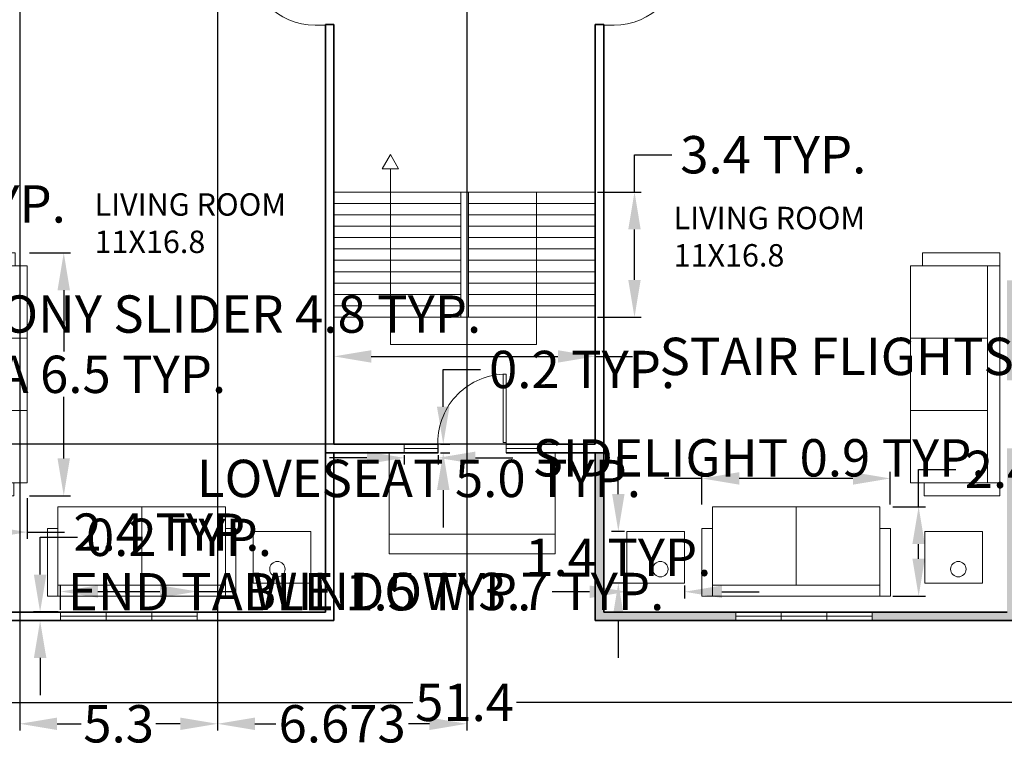
# Model space of a CAD drawing. Units: metres. Extents: x 25.1 to 96.1, y 24.3 to 71.3.
# Tile 2 of 5: x 45.8 to 72.2, y 24.3 to 43.8. Entities that reach past the tile are written whole.
import ezdxf

# ---------------------------------------------------------------- set-up
doc = ezdxf.new("R2010")
doc.units = ezdxf.units.M
doc.header["$MEASUREMENT"] = 0
for name, color, linetype, lineweight in [('A-ANNO-SYMB', 7, 'Continuous', 13), ('A-AREA-IDEN', 1, 'Continuous', 18), ('A-FLOR-STRS', 7, 'Continuous', 18), ('A-GLAZ', 4, 'Continuous', 18), ('A-WALL', 7, 'Continuous', 35), ('A-WALL-PATT', 252, 'Continuous', 13), ('dimension', 80, 'Continuous', 18), ('door', 17, 'Continuous', 18), ('furniture', 163, 'Continuous', 18)]:
    doc.layers.add(name, color=color, linetype=linetype, lineweight=lineweight)
doc.styles.get("Standard").update_dxf_attribs({"font": 'arial.ttf'})
doc.dimstyles.get("Standard").update_dxf_attribs({"dimtxt": 1, "dimasz": 1, "dimexe": 0.18, "dimexo": 0.0625, "dimgap": 0.09, "dimtad": 0, "dimtih": 1, "dimtoh": 1, "dimdec": 1, "dimzin": 0, "dimdsep": 46, "dimtxsty": 'Standard', "dimcen": 0.09, "dimadec": 0, "dimazin": 0, "dimtfac": 1, "dimtdec": 1, "dimtofl": 0, "dimtmove": 0, "dimatfit": 3, "dimfxl": 1, "dimtolj": 1, "dimtzin": 0, "dimarcsym": 0})

# ---------------------------------------------------------------- blocks, each defined once
blk = doc.blocks.new('s 2')
for points in [[(29.401, -17.335), (31.033, -17.335), (31.033, -18.866), (29.401, -18.866)], [(31.033, -17.335), (32.664, -17.335), (32.664, -18.866), (31.033, -18.866)], [(29.401, -19.079), (29.196, -19.079), (29.196, -17.761), (29.401, -17.761)], [(32.869, -19.079), (32.664, -19.079), (32.664, -17.761), (32.869, -17.761)], [(29.401, -18.866), (32.664, -18.866), (32.664, -19.079), (29.401, -19.079)]]:
    blk.add_lwpolyline(points, close=True)
blk = doc.blocks.new('s1')
for points in [[(27.599, -10.709), (29.238, -10.709), (29.238, -10.433), (27.599, -10.433)], [(27.863, -10.709), (27.599, -10.709), (27.599, -15.302), (27.863, -15.302)], [(27.863, -10.709), (29.494, -10.709), (29.494, -12.24), (27.863, -12.24)], [(27.863, -12.24), (29.494, -12.24), (29.494, -13.771), (27.863, -13.771)], [(27.863, -13.771), (29.494, -13.771), (29.494, -15.302), (27.863, -15.302)], [(27.599, -15.577), (29.207, -15.577), (29.207, -15.302), (27.599, -15.302)]]:
    blk.add_lwpolyline(points, close=True)
blk = doc.blocks.new('ss')
blk.add_lwpolyline([(27.948, -17.463), (29.489, -17.463), (29.489, -18.849), (27.948, -18.849)], close=True)
blk.add_circle((28.593, -18.475), 0.206)
blk = doc.blocks.new('*U22')
for p, q in [((0, 0), (0, -6)), ((40, 0), (40, -6))]:
    blk.add_line(p, q)
blk.add_lwpolyline([(0, 0), (0, 40), (1.75, 40), (1.75, 0)], close=True)
blk.add_arc((0, 0), 40, 0, 90)
blk = doc.blocks.new('*D24')
at = {"layer": 'Defpoints', "color": 0, "transparency": 16777216}
for p in [(31.99, 29.798), (83.411, 29.798), (83.411, 25.547)]:
    blk.add_point(p, dxfattribs=at)
at = {"layer": 'dimension', "color": 0, "lineweight": -2, "transparency": 16777216}
for p, q in [((31.99, 29.735), (31.99, 25.367)), ((83.411, 29.735), (83.411, 25.367)), ((32.99, 25.547), (56.314, 25.547)), ((82.411, 25.547), (59.087, 25.547))]:
    blk.add_line(p, q, dxfattribs=at)
at = {"layer": 'dimension', "color": 0, "transparency": 16777216}
for points in [[(32.99, 25.713), (32.99, 25.38), (31.99, 25.547)], [(82.411, 25.713), (82.411, 25.38), (83.411, 25.547)]]:
    blk.add_solid(points, dxfattribs=at)
at = {"layer": 'dimension', "color": 0, "transparency": 16777216, "insert": (57.7, 25.547), "char_height": 1, "attachment_point": 5}
blk.add_mtext('\\A1;51.4', dxfattribs=at)
blk = doc.blocks.new('ENTRY-SIDELIGHT')
for p, q in [((0, 0), (0, 0.23)), ((0, 0.115), (0.91, 0.115)), ((0.91, 0), (0.91, 0.23))]:
    blk.add_line(p, q)
blk = doc.blocks.new('STAIR-PAIRED-FLIGHTS')
for p, q in [((0, 3.353), (7, 3.353)), ((3.4, 3.353), (3.4, 0)), ((3.6, 3.353), (3.6, 0)), ((0, 3.048), (3.4, 3.048)), ((3.6, 3.048), (7, 3.048)), ((0, 2.743), (3.4, 2.743)), ((3.6, 2.743), (7, 2.743)), ((0, 2.438), (3.4, 2.438)), ((3.6, 2.438), (7, 2.438)), ((0, 2.133), (3.4, 2.133)), ((3.6, 2.133), (7, 2.133)), ((0, 1.829), (3.4, 1.829)), ((3.6, 1.829), (7, 1.829)), ((0, 1.524), (3.4, 1.524)), ((3.6, 1.524), (7, 1.524)), ((0, 1.219), (3.4, 1.219)), ((3.6, 1.219), (7, 1.219)), ((0, 0.914), (3.4, 0.914)), ((3.6, 0.914), (7, 0.914)), ((0, 0.609), (3.4, 0.609)), ((3.6, 0.609), (7, 0.609)), ((0, 0.305), (3.4, 0.305)), ((3.6, 0.305), (7, 0.305)), ((0, 0), (7, 0))]:
    blk.add_line(p, q)
blk = doc.blocks.new('WIN-THREE-LIGHTS')
for p, q in [((0, 0.115), (1.22, 0.115)), ((1.22, 0), (1.22, 0.23)), ((1.22, 0.115), (3.66, 0.115)), ((2.44, 0), (2.44, 0.23))]:
    blk.add_line(p, q)
blk = doc.blocks.new('*D30')
at = {"layer": 'Defpoints', "color": 0, "transparency": 16777216}
for p in [(62.049, 28.741), (62.049, 28.51), (63.591, 28.741)]:
    blk.add_point(p, dxfattribs=at)
at = {"layer": 'dimension', "color": 0, "lineweight": -2, "transparency": 16777216}
for p, q in [((61.049, 28.51), (60.049, 28.51)), ((62.049, 28.679), (62.049, 28.33)), ((63.591, 28.679), (63.591, 28.33)), ((64.591, 28.51), (65.591, 28.51))]:
    blk.add_line(p, q, dxfattribs=at)
at = {"layer": 'dimension', "color": 0, "transparency": 16777216}
for points in [[(61.049, 28.677), (61.049, 28.343), (62.049, 28.51)], [(64.591, 28.677), (64.591, 28.343), (63.591, 28.51)]]:
    blk.add_solid(points, dxfattribs=at)
at = {"layer": 'dimension', "color": 0, "transparency": 16777216, "insert": (53.282, 28.51), "char_height": 1, "attachment_point": 5}
blk.add_mtext('\\A1;END TABLE 1.5 TYP.', dxfattribs=at)
blk = doc.blocks.new('*D31')
at = {"layer": 'Defpoints', "color": 0, "transparency": 16777216}
for p in [(61.818, 30.127), (62.049, 30.127), (62.049, 28.741)]:
    blk.add_point(p, dxfattribs=at)
at = {"layer": 'dimension', "color": 0, "lineweight": -2, "transparency": 16777216}
for p, q in [((61.818, 31.127), (61.818, 32.127)), ((61.987, 30.127), (61.638, 30.127)), ((61.987, 28.741), (61.638, 28.741)), ((61.818, 27.741), (61.818, 26.741))]:
    blk.add_line(p, q, dxfattribs=at)
at = {"layer": 'dimension', "color": 0, "transparency": 16777216}
for points in [[(61.651, 31.127), (61.985, 31.127), (61.818, 30.127)], [(61.651, 27.741), (61.985, 27.741), (61.818, 28.741)]]:
    blk.add_solid(points, dxfattribs=at)
at = {"layer": 'dimension', "color": 0, "transparency": 16777216, "insert": (61.818, 29.434), "char_height": 1, "attachment_point": 5}
blk.add_mtext('\\A1;1.4 TYP.', dxfattribs=at)
blk = doc.blocks.new('*D34')
at = {"layer": 'Defpoints', "color": 0, "transparency": 16777216}
for p in [(46.002, 46.126), (50.795, 46.126), (50.795, 45.407)]:
    blk.add_point(p, dxfattribs=at)
at = {"layer": 'dimension', "color": 0, "lineweight": -2, "transparency": 16777216}
for p, q in [((46.002, 46.063), (46.002, 45.227)), ((50.795, 46.063), (50.795, 45.227)), ((47.002, 45.407), (49.795, 45.407)), ((50.795, 45.407), (51.795, 45.407))]:
    blk.add_line(p, q, dxfattribs=at)
at = {"layer": 'dimension', "color": 0, "transparency": 16777216}
for points in [[(47.002, 45.573), (47.002, 45.24), (46.002, 45.407)], [(49.795, 45.573), (49.795, 45.24), (50.795, 45.407)]]:
    blk.add_solid(points, dxfattribs=at)
at = {"layer": 'dimension', "color": 0, "transparency": 16777216, "insert": (56.117, 45.407), "char_height": 1, "attachment_point": 5}
blk.add_mtext('\\A1;TUB 4.8 TYP.', dxfattribs=at)
blk = doc.blocks.new('*D38')
at = {"layer": 'Defpoints', "color": 0, "transparency": 16777216}
for p in [(64.056, 31.545), (64.056, 30.788), (69.103, 30.788)]:
    blk.add_point(p, dxfattribs=at)
at = {"layer": 'dimension', "color": 0, "lineweight": -2, "transparency": 16777216}
for p, q in [((64.056, 30.851), (64.056, 31.725)), ((69.103, 30.851), (69.103, 31.725)), ((64.056, 31.545), (63.056, 31.545)), ((68.103, 31.545), (65.056, 31.545))]:
    blk.add_line(p, q, dxfattribs=at)
at = {"layer": 'dimension', "color": 0, "transparency": 16777216}
for points in [[(65.056, 31.712), (65.056, 31.379), (64.056, 31.545)], [(68.103, 31.712), (68.103, 31.379), (69.103, 31.545)]]:
    blk.add_solid(points, dxfattribs=at)
at = {"layer": 'dimension', "color": 0, "transparency": 16777216, "insert": (56.478, 31.545), "char_height": 1, "attachment_point": 5}
blk.add_mtext('\\A1;LOVESEAT 5.0 TYP.', dxfattribs=at)
blk = doc.blocks.new('*D39')
at = {"layer": 'Defpoints', "color": 0, "transparency": 16777216}
for p in [(69.103, 30.788), (69.861, 30.788), (69.103, 28.392)]:
    blk.add_point(p, dxfattribs=at)
at = {"layer": 'dimension', "color": 0, "lineweight": -2, "transparency": 16777216}
for p, q in [((69.861, 30.788), (69.861, 31.788)), ((69.861, 31.788), (70.861, 31.788)), ((69.166, 30.788), (70.041, 30.788)), ((69.861, 29.392), (69.861, 29.788)), ((69.166, 28.392), (70.041, 28.392))]:
    blk.add_line(p, q, dxfattribs=at)
at = {"layer": 'dimension', "color": 0, "transparency": 16777216}
for points in [[(69.694, 29.788), (70.027, 29.788), (69.861, 30.788)], [(69.694, 29.392), (70.027, 29.392), (69.861, 28.392)]]:
    blk.add_solid(points, dxfattribs=at)
at = {"layer": 'dimension', "color": 0, "transparency": 16777216, "insert": (73.587, 31.788), "char_height": 1, "attachment_point": 5}
blk.add_mtext('\\A1;2.4 TYP.', dxfattribs=at)
blk = doc.blocks.new('*D40')
at = {"layer": 'Defpoints', "color": 0, "transparency": 16777216}
for p in [(45.988, 37.586), (46.964, 37.586), (45.988, 31.082)]:
    blk.add_point(p, dxfattribs=at)
at = {"layer": 'dimension', "color": 0, "lineweight": -2, "transparency": 16777216}
for p, q in [((46.051, 37.586), (47.144, 37.586)), ((46.964, 36.586), (46.964, 34.941)), ((46.964, 32.082), (46.964, 33.727)), ((46.051, 31.082), (47.144, 31.082))]:
    blk.add_line(p, q, dxfattribs=at)
at = {"layer": 'dimension', "color": 0, "transparency": 16777216}
for points in [[(46.797, 36.586), (47.13, 36.586), (46.964, 37.586)], [(46.797, 32.082), (47.13, 32.082), (46.964, 31.082)]]:
    blk.add_solid(points, dxfattribs=at)
at = {"layer": 'dimension', "color": 0, "transparency": 16777216, "insert": (46.964, 34.334), "char_height": 1, "attachment_point": 5}
blk.add_mtext('\\A1;SOFA 6.5 TYP.', dxfattribs=at)
blk = doc.blocks.new('*D41')
at = {"layer": 'Defpoints', "color": 0, "transparency": 16777216}
for p in [(43.592, 31.082), (45.988, 31.082), (45.988, 30.107)]:
    blk.add_point(p, dxfattribs=at)
at = {"layer": 'dimension', "color": 0, "lineweight": -2, "transparency": 16777216}
for p, q in [((43.592, 31.02), (43.592, 29.927)), ((45.988, 31.02), (45.988, 29.927)), ((44.592, 30.107), (44.988, 30.107)), ((45.988, 30.107), (46.988, 30.107))]:
    blk.add_line(p, q, dxfattribs=at)
at = {"layer": 'dimension', "color": 0, "transparency": 16777216}
for points in [[(44.592, 30.273), (44.592, 29.94), (43.592, 30.107)], [(44.988, 30.273), (44.988, 29.94), (45.988, 30.107)]]:
    blk.add_solid(points, dxfattribs=at)
at = {"layer": 'dimension', "color": 0, "transparency": 16777216, "insert": (49.714, 30.107), "char_height": 1, "attachment_point": 5}
blk.add_mtext('\\A1;2.4 TYP.', dxfattribs=at)
blk = doc.blocks.new('*D58')
at = {"layer": 'Defpoints', "color": 0, "transparency": 16777216}
for p in [(51.177, 45.965), (53.877, 45.965), (53.877, 45.56)]:
    blk.add_point(p, dxfattribs=at)
at = {"layer": 'dimension', "color": 0, "lineweight": -2, "transparency": 16777216}
for p, q in [((51.177, 45.903), (51.177, 45.38)), ((53.877, 45.903), (53.877, 45.38)), ((52.177, 45.56), (52.877, 45.56)), ((53.877, 45.56), (54.877, 45.56))]:
    blk.add_line(p, q, dxfattribs=at)
at = {"layer": 'dimension', "color": 0, "transparency": 16777216}
for points in [[(52.177, 45.727), (52.177, 45.394), (51.177, 45.56)], [(52.877, 45.727), (52.877, 45.394), (53.877, 45.56)]]:
    blk.add_solid(points, dxfattribs=at)
at = {"layer": 'dimension', "color": 0, "transparency": 16777216, "insert": (60.81, 45.56), "char_height": 1, "attachment_point": 5}
blk.add_mtext('\\A1;CABINET 2.7 TYP.', dxfattribs=at)
blk = doc.blocks.new('*D68')
at = {"layer": 'Defpoints', "color": 0, "transparency": 16777216}
for p in [(56.082, 32.234), (56.992, 32.234), (56.992, 32.097)]:
    blk.add_point(p, dxfattribs=at)
at = {"layer": 'dimension', "color": 0, "lineweight": -2, "transparency": 16777216}
for p, q in [((55.082, 32.097), (54.082, 32.097)), ((56.082, 32.171), (56.082, 31.917)), ((56.992, 32.171), (56.992, 31.917)), ((57.992, 32.097), (58.992, 32.097))]:
    blk.add_line(p, q, dxfattribs=at)
at = {"layer": 'dimension', "color": 0, "transparency": 16777216}
for points in [[(55.082, 32.264), (55.082, 31.93), (56.082, 32.097)], [(57.992, 32.264), (57.992, 31.93), (56.992, 32.097)]]:
    blk.add_solid(points, dxfattribs=at)
at = {"layer": 'dimension', "color": 0, "transparency": 16777216, "insert": (65.588, 32.097), "char_height": 1, "attachment_point": 5}
blk.add_mtext('\\A1;SIDELIGHT 0.9 TYP.', dxfattribs=at)
blk = doc.blocks.new('*D69')
at = {"layer": 'Defpoints', "color": 0, "transparency": 16777216}
for p in [(56.992, 32.464), (57.128, 32.464), (56.992, 32.234)]:
    blk.add_point(p, dxfattribs=at)
at = {"layer": 'dimension', "color": 0, "lineweight": -2, "transparency": 16777216}
for p, q in [((57.128, 33.464), (57.128, 34.464)), ((57.128, 34.464), (58.128, 34.464)), ((57.054, 32.464), (57.308, 32.464)), ((57.054, 32.234), (57.308, 32.234)), ((57.128, 31.234), (57.128, 30.234))]:
    blk.add_line(p, q, dxfattribs=at)
at = {"layer": 'dimension', "color": 0, "transparency": 16777216}
for points in [[(56.961, 33.464), (57.295, 33.464), (57.128, 32.464)], [(56.961, 31.234), (57.295, 31.234), (57.128, 32.234)]]:
    blk.add_solid(points, dxfattribs=at)
at = {"layer": 'dimension', "color": 0, "transparency": 16777216, "insert": (60.846, 34.464), "char_height": 1, "attachment_point": 5}
blk.add_mtext('\\A1;0.2 TYP.', dxfattribs=at)
blk = doc.blocks.new('*D72')
at = {"layer": 'Defpoints', "color": 0, "transparency": 16777216}
for p in [(54.201, 35.864), (61.201, 35.864), (61.201, 34.814)]:
    blk.add_point(p, dxfattribs=at)
at = {"layer": 'dimension', "color": 0, "lineweight": -2, "transparency": 16777216}
for p, q in [((54.201, 35.801), (54.201, 34.634)), ((61.201, 35.801), (61.201, 34.634)), ((55.201, 34.814), (60.201, 34.814)), ((61.201, 34.814), (62.201, 34.814))]:
    blk.add_line(p, q, dxfattribs=at)
at = {"layer": 'dimension', "color": 0, "transparency": 16777216}
for points in [[(55.201, 34.98), (55.201, 34.647), (54.201, 34.814)], [(60.201, 34.98), (60.201, 34.647), (61.201, 34.814)]]:
    blk.add_solid(points, dxfattribs=at)
at = {"layer": 'dimension', "color": 0, "transparency": 16777216, "insert": (70.311, 34.814), "char_height": 1, "attachment_point": 5}
blk.add_mtext('\\A1;STAIR FLIGHTS 7.0 TYP.', dxfattribs=at)
blk = doc.blocks.new('*D73')
at = {"layer": 'Defpoints', "color": 0, "transparency": 16777216}
for p in [(61.201, 39.216), (62.251, 39.216), (61.201, 35.864)]:
    blk.add_point(p, dxfattribs=at)
at = {"layer": 'dimension', "color": 0, "lineweight": -2, "transparency": 16777216}
for p, q in [((62.251, 39.216), (62.251, 40.216)), ((62.251, 40.216), (63.251, 40.216)), ((61.263, 39.216), (62.431, 39.216)), ((62.251, 36.864), (62.251, 38.216)), ((61.263, 35.864), (62.431, 35.864))]:
    blk.add_line(p, q, dxfattribs=at)
at = {"layer": 'dimension', "color": 0, "transparency": 16777216}
for points in [[(62.084, 38.216), (62.417, 38.216), (62.251, 39.216)], [(62.084, 36.864), (62.417, 36.864), (62.251, 35.864)]]:
    blk.add_solid(points, dxfattribs=at)
at = {"layer": 'dimension', "color": 0, "transparency": 16777216, "insert": (65.968, 40.216), "char_height": 1, "attachment_point": 5}
blk.add_mtext('\\A1;3.4 TYP.', dxfattribs=at)
blk = doc.blocks.new('*D74')
at = {"layer": 'Defpoints', "color": 0, "transparency": 16777216}
for p in [(50.54, 28.517), (46.88, 27.968), (50.54, 27.968)]:
    blk.add_point(p, dxfattribs=at)
at = {"layer": 'dimension', "color": 0, "lineweight": -2, "transparency": 16777216}
for p, q in [((46.88, 28.03), (46.88, 28.697)), ((47.88, 28.517), (49.54, 28.517)), ((50.54, 28.03), (50.54, 28.697)), ((50.54, 28.517), (51.54, 28.517))]:
    blk.add_line(p, q, dxfattribs=at)
at = {"layer": 'dimension', "color": 0, "transparency": 16777216}
for points in [[(47.88, 28.683), (47.88, 28.35), (46.88, 28.517)], [(49.54, 28.683), (49.54, 28.35), (50.54, 28.517)]]:
    blk.add_solid(points, dxfattribs=at)
at = {"layer": 'dimension', "color": 0, "transparency": 16777216, "insert": (57.538, 28.517), "char_height": 1, "attachment_point": 5}
blk.add_mtext('\\A1;WINDOW 3.7 TYP.', dxfattribs=at)
blk = doc.blocks.new('*D75')
at = {"layer": 'Defpoints', "color": 0, "transparency": 16777216}
for p in [(46.331, 27.968), (46.88, 27.968), (46.88, 27.738)]:
    blk.add_point(p, dxfattribs=at)
at = {"layer": 'dimension', "color": 0, "lineweight": -2, "transparency": 16777216}
for p, q in [((46.331, 28.968), (46.331, 29.968)), ((46.331, 29.968), (47.331, 29.968)), ((46.818, 27.968), (46.151, 27.968)), ((46.818, 27.738), (46.151, 27.738)), ((46.331, 26.738), (46.331, 25.738))]:
    blk.add_line(p, q, dxfattribs=at)
at = {"layer": 'dimension', "color": 0, "transparency": 16777216}
for points in [[(46.165, 28.968), (46.498, 28.968), (46.331, 27.968)], [(46.165, 26.738), (46.498, 26.738), (46.331, 27.738)]]:
    blk.add_solid(points, dxfattribs=at)
at = {"layer": 'dimension', "color": 0, "transparency": 16777216, "insert": (50.049, 29.968), "char_height": 1, "attachment_point": 5}
blk.add_mtext('\\A1;0.2 TYP.', dxfattribs=at)
blk = doc.blocks.new('*D76')
at = {"layer": 'Defpoints', "color": 0, "transparency": 16777216}
for p in [(35.294, 36.668), (40.091, 36.668), (40.091, 35.948)]:
    blk.add_point(p, dxfattribs=at)
at = {"layer": 'dimension', "color": 0, "lineweight": -2, "transparency": 16777216}
for p, q in [((35.294, 36.605), (35.294, 35.768)), ((40.091, 36.605), (40.091, 35.768)), ((36.294, 35.948), (39.091, 35.948)), ((40.091, 35.948), (41.091, 35.948))]:
    blk.add_line(p, q, dxfattribs=at)
at = {"layer": 'dimension', "color": 0, "transparency": 16777216}
for points in [[(36.294, 36.115), (36.294, 35.781), (35.294, 35.948)], [(39.091, 36.115), (39.091, 35.781), (40.091, 35.948)]]:
    blk.add_solid(points, dxfattribs=at)
at = {"layer": 'dimension', "color": 0, "transparency": 16777216, "insert": (50.036, 35.948), "char_height": 1, "attachment_point": 5}
blk.add_mtext('\\A1;BALCONY SLIDER 4.8 TYP.', dxfattribs=at)
blk = doc.blocks.new('*D77')
at = {"layer": 'Defpoints', "color": 0, "transparency": 16777216}
for p in [(40.091, 36.898), (40.091, 36.668), (40.81, 36.898)]:
    blk.add_point(p, dxfattribs=at)
at = {"layer": 'dimension', "color": 0, "lineweight": -2, "transparency": 16777216}
for p, q in [((40.81, 37.898), (40.81, 38.898)), ((40.81, 38.898), (41.81, 38.898)), ((40.153, 36.898), (40.99, 36.898)), ((40.153, 36.668), (40.99, 36.668)), ((40.81, 35.668), (40.81, 34.668))]:
    blk.add_line(p, q, dxfattribs=at)
at = {"layer": 'dimension', "color": 0, "transparency": 16777216}
for points in [[(40.643, 37.898), (40.977, 37.898), (40.81, 36.898)], [(40.643, 35.668), (40.977, 35.668), (40.81, 36.668)]]:
    blk.add_solid(points, dxfattribs=at)
at = {"layer": 'dimension', "color": 0, "transparency": 16777216, "insert": (44.528, 38.898), "char_height": 1, "attachment_point": 5}
blk.add_mtext('\\A1;0.2 TYP.', dxfattribs=at)
blk = doc.blocks.new('*D78')
at = {"layer": 'Defpoints', "color": 0, "transparency": 16777216}
for p in [(45.784, 45.898), (51.084, 45.898), (51.084, 24.973)]:
    blk.add_point(p, dxfattribs=at)
at = {"layer": 'dimension', "color": 0, "lineweight": -2, "transparency": 16777216}
for p, q in [((45.784, 45.835), (45.784, 24.793)), ((51.084, 45.835), (51.084, 24.793)), ((46.784, 24.973), (47.434, 24.973)), ((50.084, 24.973), (49.434, 24.973))]:
    blk.add_line(p, q, dxfattribs=at)
at = {"layer": 'dimension', "color": 0, "transparency": 16777216}
for points in [[(46.784, 25.139), (46.784, 24.806), (45.784, 24.973)], [(50.084, 25.139), (50.084, 24.806), (51.084, 24.973)]]:
    blk.add_solid(points, dxfattribs=at)
at = {"layer": 'dimension', "color": 0, "transparency": 16777216, "insert": (48.434, 24.973), "char_height": 1, "attachment_point": 5}
blk.add_mtext('\\A1;5.3', dxfattribs=at)
blk = doc.blocks.new('*D79')
at = {"layer": 'Defpoints', "color": 0, "transparency": 16777216}
for p in [(51.084, 45.898), (57.757, 46.048), (57.757, 24.973)]:
    blk.add_point(p, dxfattribs=at)
at = {"layer": 'dimension', "color": 0, "lineweight": -2, "transparency": 16777216}
for p, q in [((57.757, 45.985), (57.757, 24.793)), ((51.084, 45.835), (51.084, 24.793)), ((52.084, 24.973), (52.641, 24.973)), ((56.757, 24.973), (56.201, 24.973))]:
    blk.add_line(p, q, dxfattribs=at)
at = {"layer": 'dimension', "color": 0, "transparency": 16777216}
for points in [[(52.084, 25.139), (52.084, 24.806), (51.084, 24.973)], [(56.757, 25.139), (56.757, 24.806), (57.757, 24.973)]]:
    blk.add_solid(points, dxfattribs=at)
at = {"layer": 'dimension', "color": 0, "transparency": 16777216, "insert": (54.421, 24.973), "char_height": 1, "attachment_point": 5}
blk.add_mtext('\\A1;6.673', dxfattribs=at)
blk = doc.blocks.new('*D84')
at = {"layer": 'Defpoints', "color": 0, "transparency": 16777216}
for p in [(29.225, 45.898), (61.201, 45.898), (61.201, 32.464)]:
    blk.add_point(p, dxfattribs=at)
at = {"layer": 'dimension', "color": 0, "lineweight": -2, "transparency": 16777216}
for p, q in [((61.138, 45.898), (29.045, 45.898)), ((29.225, 44.898), (29.225, 39.781)), ((29.225, 33.464), (29.225, 38.58)), ((61.138, 32.464), (29.045, 32.464))]:
    blk.add_line(p, q, dxfattribs=at)
at = {"layer": 'dimension', "color": 0, "transparency": 16777216}
for points in [[(29.059, 44.898), (29.392, 44.898), (29.225, 45.898)], [(29.059, 33.464), (29.392, 33.464), (29.225, 32.464)]]:
    blk.add_solid(points, dxfattribs=at)
at = {"layer": 'dimension', "color": 0, "transparency": 16777216, "insert": (29.225, 39.181), "char_height": 1, "attachment_point": 5}
blk.add_mtext('\\A1;13.434', dxfattribs=at)

msp = doc.modelspace()

# ---------------------------------------------------------------- hatches: boundary and pattern name
at = {"layer": 'A-WALL-PATT'}
h = msp.add_hatch(color=256, dxfattribs=at)
h.dxf.hatch_style = 1
h.paths.add_polyline_path([(83.4108, 47.8784), (83.1808, 47.8784), (83.1808, 46.0016), (81.3508, 46.0016), (81.3508, 45.8516), (83.1808, 45.8516), (83.1808, 36.8516), (81.298, 36.8516), (81.298, 36.6216), (83.3108, 36.6216), (83.3108, 29.8975), (72.3808, 29.8975), (72.3808, 32.3495), (72.2308, 32.3495), (72.2308, 27.9675), (68.6208, 27.9675), (68.6208, 27.7375), (72.3808, 27.7375), (72.3808, 29.7975), (83.4108, 29.7975), (83.4108, 36.6216)])
h.paths.add_polyline_path([(76.5012, 36.8516), (72.2308, 36.8516), (72.2308, 34.1695), (72.3808, 34.1695), (72.3808, 36.6216), (76.5012, 36.6216)], flags=17)
h.paths.add_polyline_path([(61.4308, 32.2335), (61.2008, 32.2335), (61.2008, 27.7375), (61.4308, 27.7375), (64.9608, 27.7375), (64.9608, 27.9675), (61.4308, 27.9675)])

# ---------------------------------------------------------------- linework, layer by layer
at = {"layer": 'A-ANNO-SYMB'}
for p, q in [((55.4889, 39.8342), (55.7137, 40.2259)), ((55.7137, 40.2259), (55.9307, 39.8342)), ((55.7137, 39.8342), (55.4889, 39.8342)), ((55.7137, 35.1316), (55.7137, 39.8342)), ((55.9307, 39.8342), (55.7137, 39.8342)), ((59.6234, 39.2163), (59.6234, 35.1316)), ((59.6234, 35.1316), (55.7137, 35.1316))]:
    msp.add_line(p, q, dxfattribs=at)
at = {"layer": 'A-FLOR-STRS'}
msp.add_line((55.678, 30.055), (60.1254, 30.055), dxfattribs=at)
msp.add_lwpolyline([(58.8117, 32.2335), (60.1254, 32.2335), (60.1254, 29.5253), (55.678, 29.5253), (55.678, 32.2335), (56.9917, 32.2335)], dxfattribs=at)
at = {"layer": 'A-GLAZ'}
for p, q in [((46.8805, 27.7375), (46.8805, 27.9675)), ((50.5405, 27.7375), (50.5405, 27.9675)), ((64.9608, 27.7375), (64.9608, 27.9675)), ((68.6208, 27.7375), (68.6208, 27.9675))]:
    msp.add_line(p, q, dxfattribs=at)
at = {"layer": 'A-WALL'}
for p, q in [((53.9708, 43.7013), (53.9708, 27.9675)), ((53.9708, 43.7013), (54.2008, 43.7013)), ((54.2008, 43.7013), (54.2008, 32.4635)), ((61.2008, 43.7013), (61.2008, 32.4635)), ((61.2008, 43.7013), (61.4308, 43.7013)), ((61.4308, 43.7013), (61.4308, 27.9675)), ((54.2008, 32.4635), (56.9917, 32.4635)), ((58.8117, 32.4635), (61.2008, 32.4635)), ((53.9708, 32.2335), (56.9917, 32.2335)), ((54.2008, 32.2335), (54.2008, 27.7375)), ((58.8117, 32.2335), (61.4308, 32.2335)), ((61.2008, 32.2335), (61.2008, 27.7375)), ((53.9708, 27.9675), (43.3702, 27.9675)), ((61.4308, 27.9675), (72.2308, 27.9675)), ((54.2008, 27.7375), (43.2202, 27.7375)), ((61.2008, 27.7375), (72.3808, 27.7375)), ((61.2008, 27.7375), (61.4308, 27.7375))]:
    msp.add_line(p, q, dxfattribs=at)

# ---------------------------------------------------------------- block references
at = {"layer": 'A-FLOR-STRS'}
msp.add_blockref('STAIR-PAIRED-FLIGHTS', (54.201, 35.8638), dxfattribs=at)
at = {"layer": 'A-GLAZ'}
for name, p in [('ENTRY-SIDELIGHT', (56.082, 32.234)), ('WIN-THREE-LIGHTS', (46.88, 27.738)), ('WIN-THREE-LIGHTS', (64.9603, 27.738))]:
    msp.add_blockref(name, p, dxfattribs=at)
at = {"layer": 'A-GLAZ', "rotation": 180}
msp.add_blockref('ENTRY-SIDELIGHT', (59.7213, 32.463), dxfattribs=at)
at = {"layer": 'door'}
for p, xscale, yscale, zscale, rotation in [((53.6991, 45.5013), -0.0452901221034344, 0.0452901221034344, 0.0452901221034344, 90), ((61.7025, 45.5013), 0.0452901221034344, 0.0452901221034344, 0.0452901221034344, 270), ((58.8117, 32.5079), -0.045724569271109, 0.045724569271109, 0.045724569271109, 359.9999999999992)]:
    msp.add_blockref('*U22', p, dxfattribs=dict(at, xscale=xscale, yscale=yscale, zscale=zscale, rotation=rotation))
at = {"layer": 'furniture'}
for name, p, xscale, yscale, zscale in [('s1', (8.6961, 50.7774), 1.264373167528455, 1.264373167528455, 1.264373167528455), ('s1', (106.9355, 50.7774), -1.264373167528455, 1.264373167528455, 1.264373167528455), ('s 2', (6.4085, 54.6089), 1.374151064391452, 1.374151064391452, 1.374151064391452), ('s 2', (109.2231, 54.6089), -1.374151064391452, 1.374151064391452, 1.374151064391452)]:
    msp.add_blockref(name, p, dxfattribs=dict(at, xscale=xscale, yscale=yscale, zscale=zscale))
msp.add_blockref('ss', (24.0929, 47.5898), dxfattribs=at)
at = {"layer": 'furniture', "xscale": -1}
for p in [(91.5387, 47.5898), (99.5175, 47.5898)]:
    msp.add_blockref('ss', p, dxfattribs=at)

# ---------------------------------------------------------------- texts
at = {"layer": 'A-AREA-IDEN', "char_height": 0.6, "attachment_point": 1}
for width, insert in [(7.701055, (47.7879, 39.1836)), (8.440404, (63.2975, 38.8214))]:
    msp.add_mtext_dynamic_manual_height_columns('LIVING ROOM\\P11X16.8', width=width, gutter_width=1, heights=[0], dxfattribs=dict(at, insert=insert))

# ---------------------------------------------------------------- dimensions: what is measured, and where the dimension line sits
at = {"layer": 'dimension'}
for base, p1, p2, text, picture, middle in [((50.795, 45.4068), (46.0015, 46.1258), (50.795, 46.1258), 'TUB <> TYP.', '*D34', (56.1166, 45.4068)), ((53.8766, 45.5602), (51.1766, 45.9652), (53.8766, 45.9652), 'CABINET <> TYP.', '*D58', (60.8101, 45.5602)), ((40.0906, 35.948), (35.2938, 36.6675), (40.0906, 36.6675), 'BALCONY SLIDER <> TYP.', '*D76', (50.036, 35.948)), ((61.2008, 34.8135), (54.2008, 35.8635), (61.2008, 35.8635), 'STAIR FLIGHTS <> TYP.', '*D72', (70.3109, 34.8135)), ((56.9917, 32.097), (56.0817, 32.2335), (56.9917, 32.2335), 'SIDELIGHT <> TYP.', '*D68', (65.5885, 32.097)), ((45.9881, 30.1065), (43.5915, 31.0821), (45.9881, 31.0821), '<> TYP.', '*D41', (49.7145, 30.1065)), ((50.5405, 28.5165), (46.8805, 27.9675), (50.5405, 27.9675), 'WINDOW <> TYP.', '*D74', (57.5377, 28.5165))]:
    dim = msp.add_linear_dim(base=base, p1=p1, p2=p2, text=text, dimstyle='Standard', override={"dimdec": 1, "dimlfac": 1, "dimrnd": 0, "dimzin": 0, "dimdsep": 46, "dimlunit": 2}, dxfattribs=at)
    dim.commit()
    dim.dimension.update_dxf_attribs({"geometry": picture, "text_midpoint": middle})
dim = msp.add_linear_dim(base=(29.2252, 45.8975), p1=(61.2008, 32.4635), p2=(61.2008, 45.8975), angle=90, dimstyle='Standard', override={"dimdec": 3, "dimlfac": 1, "dimrnd": 0, "dimzin": 0, "dimdsep": 46, "dimlunit": 2}, dxfattribs=at)
dim.commit()
dim.dimension.update_dxf_attribs({"geometry": '*D84', "text_midpoint": (29.2252, 39.1805)})
for base, p1, p2, override, picture, middle in [((51.0841, 24.9725), (45.7841, 45.8975), (51.0841, 45.8975), {"dimdec": 1, "dimlfac": 1, "dimrnd": 0, "dimzin": 0, "dimdsep": 46, "dimlunit": 2}, '*D78', (48.4341, 24.9725)), ((57.7574, 24.9725), (51.0841, 45.8975), (57.7574, 46.0475), {"dimdec": 3, "dimlfac": 1, "dimrnd": 0, "dimzin": 0, "dimdsep": 46, "dimlunit": 2}, '*D79', (54.4208, 24.9725)), ((83.4108, 25.5466), (31.9902, 29.7975), (83.4108, 29.7975), {"dimclrd": 0, "dimclre": 0, "dimclrt": 0}, '*D24', (57.7005, 25.5466))]:
    dim = msp.add_linear_dim(base=base, p1=p1, p2=p2, dimstyle='Standard', override=override, dxfattribs=at)
    dim.commit()
    dim.dimension.update_dxf_attribs({"geometry": picture, "text_midpoint": middle})
for base, p1, p2, angle, text, picture, middle in [((62.2508, 39.2163), (61.2008, 35.8635), (61.2008, 39.2163), 90, '<> TYP.', '*D73', (65.9683, 40.2163)), ((40.8101, 36.8975), (40.0906, 36.6675), (40.0906, 36.8975), 90, '<> TYP.', '*D77', (44.528, 38.8975)), ((46.9636, 37.5858), (45.9881, 31.0821), (45.9881, 37.5858), 90, 'SOFA <> TYP.', '*D40', (46.9636, 34.3339)), ((57.1282, 32.4635), (56.9917, 32.2335), (56.9917, 32.4635), 90, '<> TYP.', '*D69', (60.8461, 34.4635)), ((64.0556, 31.5452), (69.1034, 30.788), (64.0556, 30.788), 180, 'LOVESEAT <> TYP.', '*D38', (56.4779, 31.5452)), ((69.8605, 30.788), (69.1034, 28.392), (69.1034, 30.788), 90, '<> TYP.', '*D39', (73.587, 31.788)), ((61.8179, 30.1269), (62.0492, 28.7411), (62.0492, 30.1269), 90, '<> TYP.', '*D31', (61.8179, 29.434)), ((62.0492, 28.5099), (63.5911, 28.7411), (62.0492, 28.7411), 180, 'END TABLE <> TYP.', '*D30', (53.2819, 28.5099)), ((46.3315, 27.9675), (46.8805, 27.7375), (46.8805, 27.9675), 90, '<> TYP.', '*D75', (50.0494, 29.9675))]:
    dim = msp.add_linear_dim(base=base, p1=p1, p2=p2, angle=angle, text=text, dimstyle='Standard', override={"dimdec": 1, "dimlfac": 1, "dimrnd": 0, "dimzin": 0, "dimdsep": 46, "dimlunit": 2}, dxfattribs=at)
    dim.commit()
    dim.dimension.update_dxf_attribs({"geometry": picture, "text_midpoint": middle})

doc.saveas('drawing.dxf')
